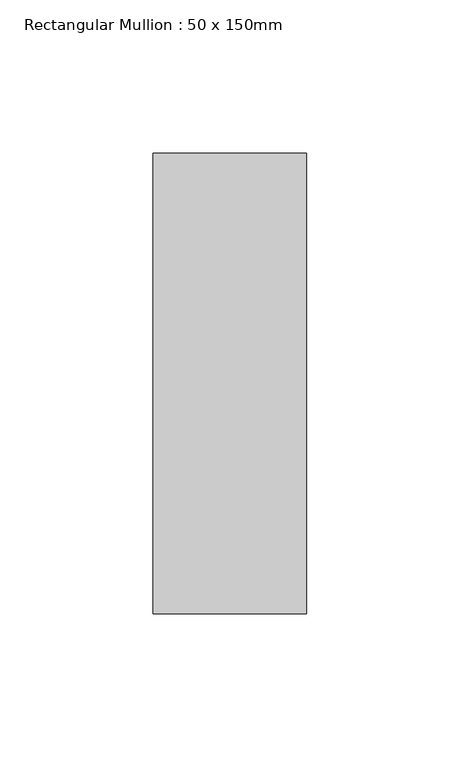
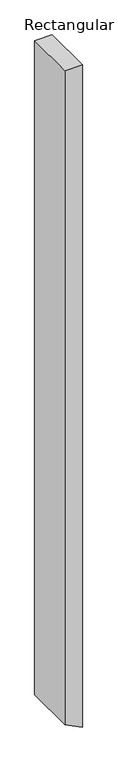
"""IFC4 building model written with IfcOpenShell, lengths in millimetres: member geometry, Rectangular Mullion : 50 x 150mm."""

from ifc_helpers import new_model, si_unit, frame, origin, place, context, project, spatial, polyline, outline, extrude, source, transform, mapped, element, save


def rectangular_mullion_50_x_150mm_0164b494(model_context):
    return source(origin(), model_context, "Body", "SweptSolid", [
        extrude(outline(polyline([(0.0, 0.0), (0.0, -50.0), (-1984.0339089, -50.0), (-2010.0622615, 0.0), (0.0, 0.0)])), frame((0.0, -75.0, 0.0), z_axis=(0.0, 1.0, 0.0), x_axis=(0.0, 0.0, 1.0)), (0.0, 0.0, 1.0), 150.0),
    ])


if __name__ == "__main__":
    model = new_model("IFC4")
    model_context = context("Model", 3, world=origin())
    ifc_project = project(units=[si_unit("LENGTHUNIT", "METRE", prefix="MILLI")], contexts=[model_context])
    site = spatial("IfcSite", under=ifc_project)
    building = spatial("IfcBuilding", under=site)
    placement = place(None, origin())
    rectangular_mullion_50_x_150mm_shape = rectangular_mullion_50_x_150mm_0164b494(model_context)
    element("IfcMember", 1, ObjectType="Rectangular Mullion : 50 x 150mm", at=placement, inside=building, context=model_context, shape_type="MappedRepresentation", body=[
        mapped(rectangular_mullion_50_x_150mm_shape, transform((0.0, 0.0, 0.0), x_axis=(1.0, 0.0, 0.0), y_axis=(0.0, 1.0, 0.0), z_axis=(0.0, 0.0, 1.0))),
    ])
    save(model, "model.ifc")

# Revit data of these elements
# Type "Rectangular Mullion : 50 x 150mm"
#   built-in parameter 1007304 = 0.492126 (stored number, unit not read)
#   built-in parameter 1007301 = 0.082021 (stored number, unit not read)
#   built-in parameter 1007300 = 0.082021 (stored number, unit not read)
# Element 1 (IfcMember, "Rectangular Mullion : 50 x 150mm")
#   Materials on its faces: "Aluminium"
# Materials
#   "Aluminium": class "Metal", colour RGB 247 247 247, transparency 0, Description = "Aluminium 6061", Cost = 0
